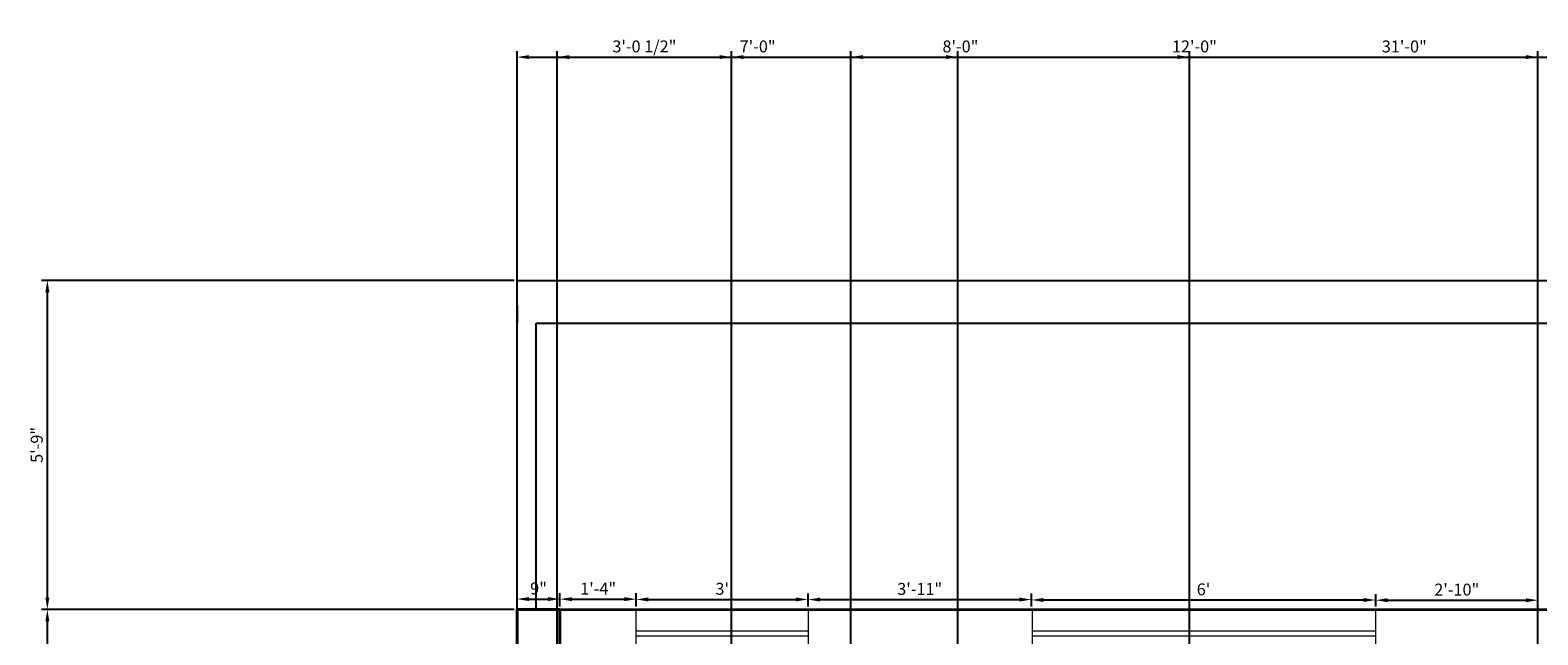
# Model space of a CAD drawing. Units: inches. Extents: x 1624 to 3956, y 1589 to 5028.
# Tile 10 of 16: x 1627 to 1943, y 2490 to 2617. Entities that reach past the tile are written whole.
import ezdxf

# ---------------------------------------------------------------- set-up
doc = ezdxf.new("R2010")
doc.units = ezdxf.units.IN
for name, color, linetype, lineweight in [('A-ANNO-DIMS', 2, 'Continuous', 13), ('A-COLS', 1, 'Continuous', 40), ('A-GLAZ', 4, 'Continuous', 18), ('A-WALL', 7, 'Continuous', 35), ('C-PROP', 7, 'Continuous', 25)]:
    doc.layers.add(name, color=color, linetype=linetype, lineweight=lineweight)
doc.styles.get("Standard").update_dxf_attribs({"font": 'arial.ttf'})
doc.dimstyles.new('Copy of ISO-25', dxfattribs={"dimtxt": 2.5, "dimasz": 2.5, "dimexe": 1.25, "dimexo": 0.625, "dimtad": 1, "dimdec": 1, "dimlunit": 4, "dimtxsty": 'Standard', "dimcen": 2.5, "dimadec": 0, "dimazin": 0, "dimtfac": 1, "dimtdec": 1, "dimtmove": 0, "dimatfit": 3, "dimfxl": 1, "dimarcsym": 0})

# ---------------------------------------------------------------- blocks, each defined once
blk = doc.blocks.new('*D25')
at = {"layer": 'A-ANNO-DIMS', "color": 0, "lineweight": -2, "transparency": 16777216}
for p, q in [((1728.58, 2496.42), (1728.58, 2499.22)), ((1731.08, 2497.97), (1735.08, 2497.97)), ((1737.58, 2496.42), (1737.58, 2499.22))]:
    blk.add_line(p, q, dxfattribs=at)
at = {"layer": 'A-ANNO-DIMS', "color": 0, "transparency": 16777216}
for points in [[(1731.08, 2498.39), (1731.08, 2497.56), (1728.58, 2497.97)], [(1735.08, 2498.39), (1735.08, 2497.56), (1737.58, 2497.97)]]:
    blk.add_solid(points, dxfattribs=at)
at = {"layer": 'Defpoints', "color": 0, "transparency": 16777216}
for p in [(1737.58, 2497.97), (1728.58, 2495.79), (1737.58, 2495.79)]:
    blk.add_point(p, dxfattribs=at)
at = {"layer": 'A-ANNO-DIMS', "color": 0, "transparency": 16777216, "insert": (1733.08, 2499.88), "char_height": 2.5, "attachment_point": 5}
blk.add_mtext('9"', dxfattribs=at)
blk = doc.blocks.new('*D26')
at = {"layer": 'A-ANNO-DIMS', "color": 0, "lineweight": -2, "transparency": 16777216}
for p, q in [((1737.58, 2496.42), (1737.58, 2499.2)), ((1740.08, 2497.95), (1751.08, 2497.95)), ((1753.58, 2496.42), (1753.58, 2499.2))]:
    blk.add_line(p, q, dxfattribs=at)
at = {"layer": 'A-ANNO-DIMS', "color": 0, "transparency": 16777216}
for points in [[(1740.08, 2498.37), (1740.08, 2497.53), (1737.58, 2497.95)], [(1751.08, 2498.37), (1751.08, 2497.53), (1753.58, 2497.95)]]:
    blk.add_solid(points, dxfattribs=at)
at = {"layer": 'Defpoints', "color": 0, "transparency": 16777216}
for p in [(1753.58, 2497.95), (1737.58, 2495.79), (1753.58, 2495.79)]:
    blk.add_point(p, dxfattribs=at)
at = {"layer": 'A-ANNO-DIMS', "color": 0, "transparency": 16777216, "insert": (1745.58, 2499.83), "char_height": 2.5, "attachment_point": 5}
blk.add_mtext('1\'-4"', dxfattribs=at)
blk = doc.blocks.new('*D27')
at = {"layer": 'A-ANNO-DIMS', "color": 0, "lineweight": -2, "transparency": 16777216}
for p, q in [((1753.58, 2496.42), (1753.58, 2499.14)), ((1756.08, 2497.89), (1787.08, 2497.89)), ((1789.58, 2496.42), (1789.58, 2499.14))]:
    blk.add_line(p, q, dxfattribs=at)
at = {"layer": 'A-ANNO-DIMS', "color": 0, "transparency": 16777216}
for points in [[(1756.08, 2498.31), (1756.08, 2497.48), (1753.58, 2497.89)], [(1787.08, 2498.31), (1787.08, 2497.48), (1789.58, 2497.89)]]:
    blk.add_solid(points, dxfattribs=at)
at = {"layer": 'Defpoints', "color": 0, "transparency": 16777216}
for p in [(1789.58, 2497.89), (1753.58, 2495.79), (1789.58, 2495.79)]:
    blk.add_point(p, dxfattribs=at)
at = {"layer": 'A-ANNO-DIMS', "color": 0, "transparency": 16777216, "insert": (1771.58, 2499.8), "char_height": 2.5, "attachment_point": 5}
blk.add_mtext("3'", dxfattribs=at)
blk = doc.blocks.new('*D28')
at = {"layer": 'A-ANNO-DIMS', "color": 0, "lineweight": -2, "transparency": 16777216}
for p, q in [((1789.58, 2496.42), (1789.58, 2499.11)), ((1792.08, 2497.86), (1833.91, 2497.86)), ((1836.41, 2496.42), (1836.41, 2499.11))]:
    blk.add_line(p, q, dxfattribs=at)
at = {"layer": 'A-ANNO-DIMS', "color": 0, "transparency": 16777216}
for points in [[(1792.08, 2498.28), (1792.08, 2497.45), (1789.58, 2497.86)], [(1833.91, 2498.28), (1833.91, 2497.45), (1836.41, 2497.86)]]:
    blk.add_solid(points, dxfattribs=at)
at = {"layer": 'Defpoints', "color": 0, "transparency": 16777216}
for p in [(1836.41, 2497.86), (1789.58, 2495.79), (1836.41, 2495.79)]:
    blk.add_point(p, dxfattribs=at)
at = {"layer": 'A-ANNO-DIMS', "color": 0, "transparency": 16777216, "insert": (1812.99, 2499.77), "char_height": 2.5, "attachment_point": 5}
blk.add_mtext('3\'-11"', dxfattribs=at)
blk = doc.blocks.new('*D29')
at = {"layer": 'A-ANNO-DIMS', "color": 0, "lineweight": -2, "transparency": 16777216}
for p, q in [((1836.41, 2496.42), (1836.41, 2499.03)), ((1838.91, 2497.78), (1906.08, 2497.78)), ((1908.58, 2496.42), (1908.58, 2499.03))]:
    blk.add_line(p, q, dxfattribs=at)
at = {"layer": 'A-ANNO-DIMS', "color": 0, "transparency": 16777216}
for points in [[(1838.91, 2498.19), (1838.91, 2497.36), (1836.41, 2497.78)], [(1906.08, 2498.19), (1906.08, 2497.36), (1908.58, 2497.78)]]:
    blk.add_solid(points, dxfattribs=at)
at = {"layer": 'Defpoints', "color": 0, "transparency": 16777216}
for p in [(1908.58, 2497.78), (1836.41, 2495.79), (1908.58, 2495.79)]:
    blk.add_point(p, dxfattribs=at)
at = {"layer": 'A-ANNO-DIMS', "color": 0, "transparency": 16777216, "insert": (1872.49, 2499.68), "char_height": 2.5, "attachment_point": 5}
blk.add_mtext("6'", dxfattribs=at)
blk = doc.blocks.new('*D30')
at = {"layer": 'A-ANNO-DIMS', "color": 0, "lineweight": -2, "transparency": 16777216}
for p, q in [((1908.58, 2496.42), (1908.58, 2498.98)), ((1911.08, 2497.73), (1940.08, 2497.73)), ((1942.58, 2496.42), (1942.58, 2498.98))]:
    blk.add_line(p, q, dxfattribs=at)
at = {"layer": 'A-ANNO-DIMS', "color": 0, "transparency": 16777216}
for points in [[(1911.08, 2498.14), (1911.08, 2497.31), (1908.58, 2497.73)], [(1940.08, 2498.14), (1940.08, 2497.31), (1942.58, 2497.73)]]:
    blk.add_solid(points, dxfattribs=at)
at = {"layer": 'Defpoints', "color": 0, "transparency": 16777216}
for p in [(1942.58, 2497.73), (1908.58, 2495.79), (1942.58, 2495.79)]:
    blk.add_point(p, dxfattribs=at)
at = {"layer": 'A-ANNO-DIMS', "color": 0, "transparency": 16777216, "insert": (1925.58, 2499.63), "char_height": 2.5, "attachment_point": 5}
blk.add_mtext('2\'-10"', dxfattribs=at)
blk = doc.blocks.new('COLUMN-9x9')
for p, q in [((0, 0), (0, 9)), ((0, 9), (9, 9)), ((9, 9), (9, 0)), ((9, 0), (0, 0))]:
    blk.add_line(p, q)
blk = doc.blocks.new('WINDOW-36IN')
for p, q in [((0, 0), (0, 9)), ((36, 9), (36, 0)), ((0, 4.5), (36, 4.5)), ((0, 3.5), (36, 3.5))]:
    blk.add_line(p, q)
blk = doc.blocks.new('WINDOW-72IN')
for p, q in [((0, 9), (0, 0)), ((72, 0), (72, 9)), ((0, 4.5), (72, 4.5)), ((0, 3.5), (72, 3.5))]:
    blk.add_line(p, q)
blk = doc.blocks.new('*D68')
at = {"layer": 'A-ANNO-DIMS', "color": 0, "lineweight": -2, "transparency": 16777216}
for p, q in [((1728.58, 2496.42), (1728.58, 2612.84)), ((1731.08, 2611.59), (2098.08, 2611.59)), ((2100.58, 2496.42), (2100.58, 2612.84))]:
    blk.add_line(p, q, dxfattribs=at)
at = {"layer": 'A-ANNO-DIMS', "color": 0, "transparency": 16777216}
for points in [[(1731.08, 2612.01), (1731.08, 2611.18), (1728.58, 2611.59)], [(2098.08, 2612.01), (2098.08, 2611.18), (2100.58, 2611.59)]]:
    blk.add_solid(points, dxfattribs=at)
at = {"layer": 'Defpoints', "color": 0, "transparency": 16777216}
for p in [(2100.58, 2611.59), (1728.58, 2495.79), (2100.58, 2495.79)]:
    blk.add_point(p, dxfattribs=at)
at = {"layer": 'A-ANNO-DIMS', "color": 0, "transparency": 16777216, "insert": (1914.58, 2613.5), "char_height": 2.5, "attachment_point": 5}
blk.add_mtext('31\'-0"', dxfattribs=at)
blk = doc.blocks.new('*D69')
at = {"layer": 'A-ANNO-DIMS', "color": 0, "lineweight": -2, "transparency": 16777216}
for p, q in [((1727.95, 2495.79), (1628.86, 2495.79)), ((1630.11, 1775.29), (1630.11, 2493.29)), ((1726.95, 1772.79), (1628.86, 1772.79))]:
    blk.add_line(p, q, dxfattribs=at)
at = {"layer": 'A-ANNO-DIMS', "color": 0, "transparency": 16777216}
for points in [[(1629.69, 2493.29), (1630.53, 2493.29), (1630.11, 2495.79)], [(1629.69, 1775.29), (1630.53, 1775.29), (1630.11, 1772.79)]]:
    blk.add_solid(points, dxfattribs=at)
at = {"layer": 'Defpoints', "color": 0, "transparency": 16777216}
for p in [(1630.11, 2495.79), (1728.58, 2495.79), (1727.58, 1772.79)]:
    blk.add_point(p, dxfattribs=at)
at = {"layer": 'A-ANNO-DIMS', "color": 0, "transparency": 16777216, "insert": (1628.21, 2134.29), "char_height": 2.5, "attachment_point": 5, "rotation": 90}
blk.add_mtext('60\'-3"', dxfattribs=at)
blk = doc.blocks.new('*D71')
at = {"layer": 'A-ANNO-DIMS', "color": 0, "lineweight": -2, "transparency": 16777216}
for p, q in [((1727.95, 2564.79), (1628.86, 2564.79)), ((1630.11, 2498.29), (1630.11, 2562.29)), ((1727.95, 2495.79), (1628.86, 2495.79))]:
    blk.add_line(p, q, dxfattribs=at)
at = {"layer": 'A-ANNO-DIMS', "color": 0, "transparency": 16777216}
for points in [[(1629.69, 2562.29), (1630.53, 2562.29), (1630.11, 2564.79)], [(1629.69, 2498.29), (1630.53, 2498.29), (1630.11, 2495.79)]]:
    blk.add_solid(points, dxfattribs=at)
at = {"layer": 'Defpoints', "color": 0, "transparency": 16777216}
for p in [(1630.11, 2564.79), (1728.58, 2564.79), (1728.58, 2495.79)]:
    blk.add_point(p, dxfattribs=at)
at = {"layer": 'A-ANNO-DIMS', "color": 0, "transparency": 16777216, "insert": (1628.21, 2530.29), "char_height": 2.5, "attachment_point": 5, "rotation": 90}
blk.add_mtext('5\'-9"', dxfattribs=at)
blk = doc.blocks.new('*D77')
at = {"layer": 'A-ANNO-DIMS', "color": 0, "lineweight": -2, "transparency": 16777216}
for p, q in [((1798.58, 2316.42), (1798.58, 2612.84)), ((1801.08, 2611.59), (1940.08, 2611.59)), ((1942.58, 2316.42), (1942.58, 2612.84))]:
    blk.add_line(p, q, dxfattribs=at)
at = {"layer": 'A-ANNO-DIMS', "color": 0, "transparency": 16777216}
for points in [[(1801.08, 2612.01), (1801.08, 2611.18), (1798.58, 2611.59)], [(1940.08, 2612.01), (1940.08, 2611.18), (1942.58, 2611.59)]]:
    blk.add_solid(points, dxfattribs=at)
at = {"layer": 'Defpoints', "color": 0, "transparency": 16777216}
for p in [(1942.58, 2611.59), (1798.58, 2315.79), (1942.58, 2315.79)]:
    blk.add_point(p, dxfattribs=at)
at = {"layer": 'A-ANNO-DIMS', "color": 0, "transparency": 16777216, "insert": (1870.58, 2613.5), "char_height": 2.5, "attachment_point": 5}
blk.add_mtext('12\'-0"', dxfattribs=at)
blk = doc.blocks.new('*D86')
at = {"layer": 'A-ANNO-DIMS', "color": 0, "lineweight": -2, "transparency": 16777216}
for p, q in [((1737.01, 1953.42), (1737.01, 2612.84)), ((1739.51, 2611.59), (1818.51, 2611.59)), ((1821.01, 1953.42), (1821.01, 2612.84))]:
    blk.add_line(p, q, dxfattribs=at)
at = {"layer": 'A-ANNO-DIMS', "color": 0, "transparency": 16777216}
for points in [[(1739.51, 2612.01), (1739.51, 2611.18), (1737.01, 2611.59)], [(1818.51, 2612.01), (1818.51, 2611.18), (1821.01, 2611.59)]]:
    blk.add_solid(points, dxfattribs=at)
at = {"layer": 'Defpoints', "color": 0, "transparency": 16777216}
for p in [(1821.01, 2611.59), (1737.01, 1952.79), (1821.01, 1952.79)]:
    blk.add_point(p, dxfattribs=at)
at = {"layer": 'A-ANNO-DIMS', "color": 0, "transparency": 16777216, "insert": (1779.01, 2613.5), "char_height": 2.5, "attachment_point": 5}
blk.add_mtext('7\'-0"', dxfattribs=at)
blk = doc.blocks.new('*D97')
at = {"layer": 'A-ANNO-DIMS', "color": 0, "lineweight": -2, "transparency": 16777216}
for p, q in [((1773.53, 1773.42), (1773.53, 2612.84)), ((1776.03, 2611.59), (1867.03, 2611.59)), ((1869.53, 1773.42), (1869.53, 2612.84))]:
    blk.add_line(p, q, dxfattribs=at)
at = {"layer": 'A-ANNO-DIMS', "color": 0, "transparency": 16777216}
for points in [[(1776.03, 2612.01), (1776.03, 2611.18), (1773.53, 2611.59)], [(1867.03, 2612.01), (1867.03, 2611.18), (1869.53, 2611.59)]]:
    blk.add_solid(points, dxfattribs=at)
at = {"layer": 'Defpoints', "color": 0, "transparency": 16777216}
for p in [(1869.53, 2611.59), (1773.53, 1772.79), (1869.53, 1772.79)]:
    blk.add_point(p, dxfattribs=at)
at = {"layer": 'A-ANNO-DIMS', "color": 0, "transparency": 16777216, "insert": (1821.53, 2613.5), "char_height": 2.5, "attachment_point": 5}
blk.add_mtext('8\'-0"', dxfattribs=at)
blk = doc.blocks.new('*D101')
at = {"layer": 'A-ANNO-DIMS', "color": 0, "lineweight": -2, "transparency": 16777216}
for p, q in [((1737.01, 1782.42), (1737.01, 2612.84)), ((1739.51, 2611.59), (1771.03, 2611.59)), ((1773.53, 1782.42), (1773.53, 2612.84))]:
    blk.add_line(p, q, dxfattribs=at)
at = {"layer": 'A-ANNO-DIMS', "color": 0, "transparency": 16777216}
for points in [[(1739.51, 2612.01), (1739.51, 2611.18), (1737.01, 2611.59)], [(1771.03, 2612.01), (1771.03, 2611.18), (1773.53, 2611.59)]]:
    blk.add_solid(points, dxfattribs=at)
at = {"layer": 'Defpoints', "color": 0, "transparency": 16777216}
for p in [(1773.53, 2611.59), (1737.01, 1781.79), (1773.53, 1781.79)]:
    blk.add_point(p, dxfattribs=at)
at = {"layer": 'A-ANNO-DIMS', "color": 0, "transparency": 16777216, "insert": (1755.27, 2613.51), "char_height": 2.5, "attachment_point": 5}
blk.add_mtext('3\'-0 1/2"', dxfattribs=at)

msp = doc.modelspace()

# ---------------------------------------------------------------- linework, layer by layer
at = {"layer": 'A-GLAZ'}
msp.add_line((1753.58, 2495.79), (1789.58, 2495.79), dxfattribs=at)
at = {"layer": 'A-WALL'}
for p, q in [((1728.58, 2486.79), (1728.58, 2495.79)), ((1728.58, 2495.79), (1733.08, 2495.79)), ((1733.08, 2495.79), (1742.08, 2495.79)), ((1742.08, 2495.79), (1758.08, 2495.79)), ((1758.08, 2495.79), (1794.08, 2495.79)), ((1789.58, 2495.79), (1836.58, 2495.79)), ((1794.08, 2495.79), (1841.08, 2495.79)), ((1841.08, 2495.79), (1913.08, 2495.79)), ((1913.08, 2495.79), (1947.08, 2495.79))]:
    msp.add_line(p, q, dxfattribs=at)
at = {"layer": 'C-PROP'}
for p, q in [((1728.58, 2564.79), (2160.58, 2564.79)), ((1728.58, 2555.79), (1728.58, 2564.79)), ((1728.58, 2559.46), (1728.58, 2555.79)), ((1728.58, 2495.79), (1728.58, 2555.79)), ((1732.58, 2555.79), (2160.58, 2555.79)), ((1732.58, 2495.79), (1732.58, 2555.79))]:
    msp.add_line(p, q, dxfattribs=at)

# ---------------------------------------------------------------- block references
at = {"layer": 'A-COLS'}
msp.add_blockref('COLUMN-9x9', (1728.58, 2486.79), dxfattribs=at)
at = {"layer": 'A-GLAZ'}
for name, p in [('WINDOW-36IN', (1753.58, 2486.79)), ('WINDOW-72IN', (1836.58, 2486.79))]:
    msp.add_blockref(name, p, dxfattribs=at)

# ---------------------------------------------------------------- dimensions: what is measured, and where the dimension line sits
at = {"layer": 'A-ANNO-DIMS'}
for base, p1, p2, override, picture, middle in [((1773.53, 2611.59), (1737.01, 1781.79), (1773.53, 1781.79), {"dimdec": 1, "dimlfac": 1, "dimrnd": 0, "dimzin": 1, "dimdsep": 46, "dimlunit": 4, "dimfrac": 2}, '*D101', (1755.27, 2613.51)), ((2100.58, 2611.59), (1728.58, 2495.79), (2100.58, 2495.79), {"dimdec": 1, "dimlfac": 1, "dimrnd": 0, "dimzin": 1, "dimdsep": 46, "dimlunit": 4, "dimfrac": 2}, '*D68', (1914.58, 2613.5)), ((1821.01, 2611.59), (1737.01, 1952.79), (1821.01, 1952.79), {"dimdec": 1, "dimlfac": 1, "dimrnd": 0, "dimzin": 1, "dimdsep": 46, "dimlunit": 4, "dimfrac": 2}, '*D86', (1779.01, 2613.5)), ((1869.53, 2611.59), (1773.53, 1772.79), (1869.53, 1772.79), {"dimdec": 1, "dimlfac": 1, "dimrnd": 0, "dimzin": 1, "dimdsep": 46, "dimlunit": 4, "dimfrac": 2}, '*D97', (1821.53, 2613.5)), ((1942.58, 2611.59), (1798.58, 2315.79), (1942.58, 2315.79), {"dimdec": 1, "dimlfac": 1, "dimrnd": 0, "dimzin": 1, "dimdsep": 46, "dimlunit": 4, "dimfrac": 2}, '*D77', (1870.58, 2613.5)), ((1737.58, 2497.97), (1728.58, 2495.79), (1737.58, 2495.79), {"dimclrd": 0, "dimclre": 0, "dimclrt": 0}, '*D25', (1733.08, 2499.88)), ((1753.58, 2497.95), (1737.58, 2495.79), (1753.58, 2495.79), {"dimclrd": 0, "dimclre": 0, "dimclrt": 0}, '*D26', (1745.58, 2499.83)), ((1789.58, 2497.89), (1753.58, 2495.79), (1789.58, 2495.79), {"dimclrd": 0, "dimclre": 0, "dimclrt": 0}, '*D27', (1771.58, 2499.8)), ((1836.41, 2497.86), (1789.58, 2495.79), (1836.41, 2495.79), {"dimclrd": 0, "dimclre": 0, "dimclrt": 0}, '*D28', (1812.99, 2499.77)), ((1908.58, 2497.78), (1836.41, 2495.79), (1908.58, 2495.79), {"dimclrd": 0, "dimclre": 0, "dimclrt": 0}, '*D29', (1872.49, 2499.68)), ((1942.58, 2497.73), (1908.58, 2495.79), (1942.58, 2495.79), {"dimclrd": 0, "dimclre": 0, "dimclrt": 0}, '*D30', (1925.58, 2499.63))]:
    dim = msp.add_linear_dim(base=base, p1=p1, p2=p2, dimstyle='Copy of ISO-25', override=override, dxfattribs=at)
    dim.commit()
    dim.dimension.update_dxf_attribs({"geometry": picture, "text_midpoint": middle})
for base, p1, p2, picture, middle in [((1630.11, 2564.79), (1728.58, 2495.79), (1728.58, 2564.79), '*D71', (1628.21, 2530.29)), ((1630.11, 2495.79), (1727.58, 1772.79), (1728.58, 2495.79), '*D69', (1628.21, 2134.29))]:
    dim = msp.add_linear_dim(base=base, p1=p1, p2=p2, angle=90, dimstyle='Copy of ISO-25', override={"dimdec": 1, "dimlfac": 1, "dimrnd": 0, "dimzin": 1, "dimdsep": 46, "dimlunit": 4, "dimfrac": 2}, dxfattribs=at)
    dim.commit()
    dim.dimension.update_dxf_attribs({"geometry": picture, "text_midpoint": middle})

doc.saveas('drawing.dxf')
